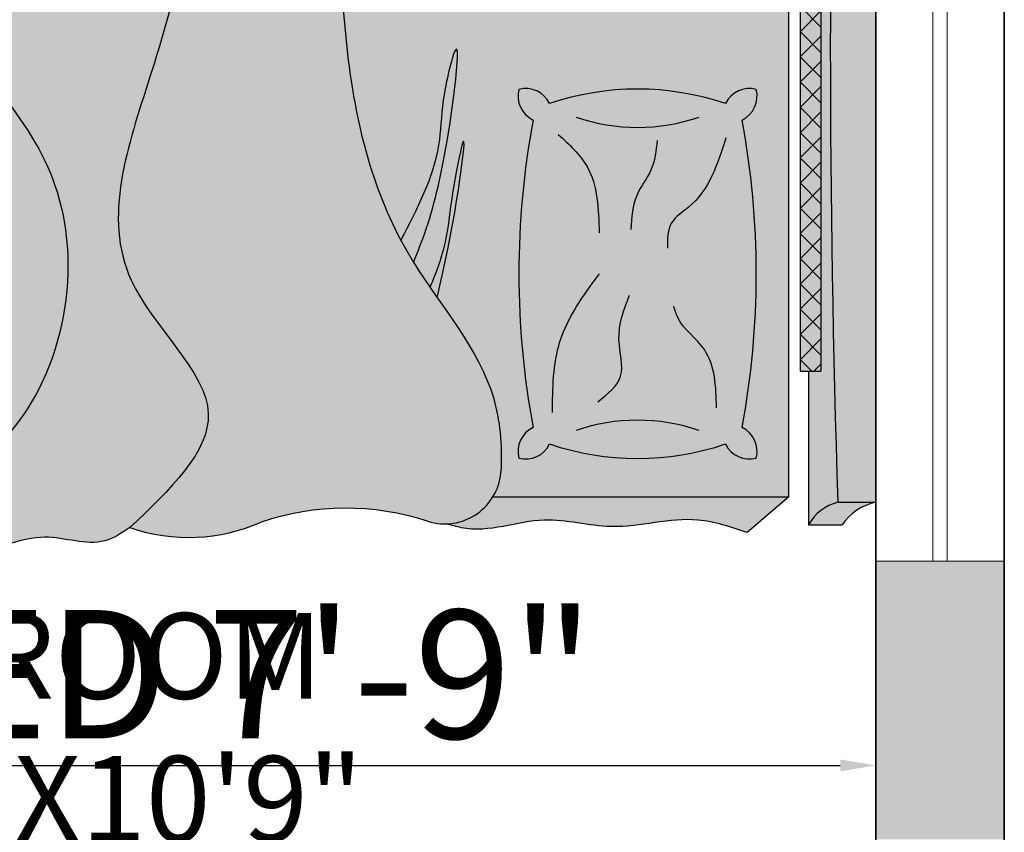
# Model space of a CAD drawing. Units: inches. Extents: x 3148 to 3962, y 1142 to 1671.
# Tile 5 of 9: x 3413 to 3482, y 1426 to 1483. Entities that reach past the tile are written whole.
import ezdxf

# ---------------------------------------------------------------- set-up
doc = ezdxf.new("R2010")
doc.units = ezdxf.units.IN
for name, color, linetype, lineweight in [('A-ANNO-DIMS', 2, 'Continuous', 18), ('A-AREA-IDEN', 7, 'Continuous', 18), ('A-FURN', 8, 'Continuous', 18), ('A-GLAZ', 4, 'Continuous', 18), ('A-WALL', 7, 'Continuous', 35), ('estofado', 7, 'Continuous', 25)]:
    doc.layers.add(name, color=color, linetype=linetype, lineweight=lineweight)
doc.layers.add('A-WALL-PATT', color=252, linetype='Continuous', lineweight=13, true_color=0x939598)
doc.styles.get("Standard").update_dxf_attribs({"font": 'arial.ttf'})
doc.dimstyles.new('ISO-25', dxfattribs={"dimtxt": 9, "dimasz": 2.5, "dimexe": 1.25, "dimexo": 0.625, "dimtad": 1, "dimdec": 1, "dimlunit": 3, "dimtxsty": 'Standard', "dimcen": 2.5, "dimadec": 0, "dimazin": 0, "dimtfac": 1, "dimtdec": 1, "dimtmove": 0, "dimatfit": 3, "dimfxl": 1, "dimarcsym": 0})

# ---------------------------------------------------------------- blocks, each defined once
blk = doc.blocks.new('Cama Box Regencia LOLA')
at = {"layer": 'estofado', "ltscale": 0.2}
h = blk.add_hatch(color=256, dxfattribs=at)
h.dxf.hatch_style = 1
h.set_gradient(color1=(139, 102, 75), color2=(43, 31, 23), one_color=1, tint=0.1299999952316284, name='CURVED')
h.paths.add_polyline_path([(0.8097611300672723, 0), (-0.8097611300671587, 0), (-0.8097611300671587, -0.0676434826297054, 0.0166383680674931), (0.8097611300672723, -0.0676434823212162)])
h = blk.add_hatch(color=256, dxfattribs=at)
h.dxf.hatch_style = 1
h.set_gradient(color1=(139, 102, 75), color2=(43, 31, 23), one_color=1, tint=0.1299999952316284)
h.paths.add_polyline_path([(0.8500000000000227, -0.0600000000000591, -0.1973270565004446), (0.8097611300672723, 0), (0.8097611300672723, -0.0676434826301033, 0.208347730813652), (0.8500000000000227, -0.1199999999998909)])
h = blk.add_hatch(color=256, dxfattribs=at)
h.dxf.hatch_style = 1
h.set_gradient(color1=(139, 102, 75), color2=(43, 31, 23), one_color=1, tint=0.1299999952316284, name='INVCURVED')
h.paths.add_polyline_path([(0.8097611299908749, -0.0676434823237742, -0.0166383680667078), (-0.8097611300671587, -0.0676434826297623, -0.2083477308153697), (-0.8500000000001364, -0.1200000000000045), (-0.5763381074484643, -0.1200000000000045), (-0.5763381074485779, -0.0977075818103117), (0.5763381073808205, -0.0977075818103117), (0.5763381073808205, -0.1200000000000045), (0.8500000000000227, -0.1200000000000045, -0.2083477318100794)])
h = blk.add_hatch(color=256, dxfattribs=at)
h.dxf.hatch_style = 1
h.set_gradient(color1=(139, 102, 75), color2=(198, 169, 149), one_color=1, tint=0.6800000071525574, name='CYLINDER')
h.paths.add_polyline_path([(0.5763381073808205, -0.0977075818103686), (-0.5763381074484643, -0.0977075818103117), (-0.5763381074485779, -0.1348263709859339), (0.5763381073808205, -0.134826370985877)])
h = blk.add_hatch(dxfattribs=at)
h.set_pattern_fill('ANSI37,_O', color=256, scale=0.01)
h.set_pattern_definition([(45, (-24.74368160026529, -44.17612681992631), (-0.0224506403026729, 0.0224506403026729), []), (135, (-24.74368160026529, -44.17612681992631), (-0.0224506403026729, -0.0224506403026729), [])])
h.paths.add_polyline_path([(0.5763381073808205, -0.0977075818103686), (-0.5763381074484643, -0.0977075818103117), (-0.5763381074485779, -0.1348263709859339), (0.5763381073808205, -0.134826370985877)])
h = blk.add_hatch(color=256, dxfattribs=at)
h.dxf.hatch_style = 1
h.set_gradient(color1=(240, 232, 219), color2=(213, 190, 154), one_color=1, tint=0.7200000286102295, name='CURVED')
edge = h.paths.add_edge_path()
edge.add_spline(control_points=[(0.343533776195045, -0.8455058148597345), (0.2879313990920309, -0.8167160606696484), (0.2054770794474052, -0.7744470032542381), (0.0954193394759386, -0.7742416952675626), (-0.0885363502328574, -0.7276964167006668), (0.2428192566063672, -0.7672518992321216), (0.345087521536243, -0.8076697826234067), (0.3825206986321063, -0.8228555492498799)], knot_values=[0.0056315103357428, 0.0056315103357428, 0.0056315103357428, 0.0056315103357428, 0.1860138916206105, 0.2660015162584448, 0.3570871810327863, 0.5963901805690979, 0.739731738908988, 0.739731738908988, 0.739731738908988, 0.739731738908988], degree=3, periodic=0)
edge.add_spline(control_points=[(0.3825206986325611, -0.8228555492497662), (0.3974221570828149, -0.8135511441712424), (0.4121061736600496, -0.8037181558521524), (0.4266849906532571, -0.7937075488799225)], knot_values=[1.358237767273279, 1.358237767273279, 1.358237767273279, 1.358237767273279, 1.409915662372559, 1.409915662372559, 1.409915662372559, 1.409915662372559], degree=3, periodic=0)
edge.add_spline(control_points=[(0.4266849905698109, -0.7937075489369932), (0.3998777739682282, -0.7821381809783361), (0.3476761897024971, -0.7634757898491671), (0.2670618099601825, -0.7565375622627358), (0.0835725072796549, -0.7192994417154637), (0.288524529784695, -0.7446405493717521), (0.4247448861246994, -0.7759943071475277), (0.4449816270193879, -0.7810438091316882)], knot_values=[0.1043639306803623, 0.1043639306803623, 0.1043639306803623, 0.1043639306803623, 0.1896363068641149, 0.2696239315019491, 0.3607095962762907, 0.6000125958126024, 0.6446217338078729, 0.6446217338078729, 0.6446217338078729, 0.6446217338078729], degree=3, periodic=0)
edge.add_spline(control_points=[(0.4449816270197289, -0.7810438091316882), (0.5029779388527232, -0.7406836481117695), (0.5966687145296419, -0.6736247633211292), (0.7071737530245628, -0.6656573253703187), (0.7517012483331201, -0.6672238302253392)], knot_values=[1.43159032281798, 1.43159032281798, 1.43159032281798, 1.43159032281798, 1.63814180148235, 1.770695287284994, 1.770695287284994, 1.770695287284994, 1.770695287284994], degree=3, periodic=0)
edge.add_arc((0.7481853615017826, -0.767162003811734), 0.0999999999999888, 58.7920033978138, 87.98512997550938, ccw=False)
edge.add_line((0.8000000000000682, -0.6816328085782289), (0.8000000000000682, -0.154802362840428))
edge.add_line((0.8000000000000682, -0.154802362840428), (-0.7999999999999546, -0.154802362840428))
edge.add_line((-0.7999999999999546, -0.154802362840428), (-0.8000000000000682, -0.7409839258539819))
edge.add_spline(control_points=[(-0.799999999999841, -0.7409839258539251), (-0.7846451382113174, -0.74846387981205), (-0.7568940913494089, -0.7651582159765554), (-0.7559936909002545, -0.8096905380045313), (-0.7049413305308008, -0.8142555457367848), (-0.7013836936888538, -0.8139988647640733)], knot_values=[0.0122267587020837, 0.0122267587020837, 0.0122267587020837, 0.0122267587020837, 0.0594720782072034, 0.1062176618094138, 0.134458043575382, 0.134458043575382, 0.134458043575382, 0.134458043575382], degree=3, periodic=0)
edge.add_spline(control_points=[(-0.7013836936890812, -0.8139988647637892), (-0.6428309483887916, -0.8132695376718857), (-0.532520673001045, -0.8118955240036598), (-0.2390712668254764, -0.6717984706609172), (-0.3892411364554391, -0.7557901092520752), (-0.4591093260188473, -0.8070101468627512), (-0.5571511178645779, -0.795652750469742), (-0.608497950975675, -0.8409486634728295), (-0.6632498050151981, -0.8266781836207997), (-0.6991149398675134, -0.8254126024436914), (-0.719552182989446, -0.8246914287938125)], knot_values=[0, 0, 0, 0, 0.2187005959148062, 0.4120203559900679, 0.4786136596093368, 0.6046444033330721, 0.6969970394608519, 0.7456449795902803, 0.7925683322559657, 0.8547274388453192, 0.8547274388453192, 0.8547274388453192, 0.8547274388453192], degree=3, periodic=0)
edge.add_spline(control_points=[(-0.7195521829781911, -0.824691428792164), (-0.7293124663336812, -0.8248308281530967), (-0.7545977292818407, -0.8216412233076653), (-0.7742556984202338, -0.794819860189591), (-0.7939222919129634, -0.7820064600295497), (-0.799999999999841, -0.7800193173443404)], knot_values=[0.1564883932805935, 0.1564883932805935, 0.1564883932805935, 0.1564883932805935, 0.184397548386913, 0.2313764834161266, 0.2505984550882281, 0.2505984550882281, 0.2505984550882281, 0.2505984550882281], degree=3, periodic=0)
edge.add_line((-0.8000000000000682, -0.7800193173444541), (-0.7999999999999546, -0.8218505664627286))
edge.add_spline(control_points=[(-0.7999999999999546, -0.8218505664625013), (-0.7938082505512511, -0.8290217081292894), (-0.7673857405620766, -0.8512914803976059), (-0.7619109683460011, -0.8661369353891359), (-0.6555700939965164, -0.8510070218793543), (-0.7139793977868294, -0.8637526923380391), (-0.7379026254519659, -0.8623504601624176), (-0.7688129786438367, -0.8813042143888196), (-0.7854260296310259, -0.8561610219318254), (-0.7961930533253962, -0.8566031243811949), (-0.7999999999999546, -0.8573491405791173)], knot_values=[0.0595743221876141, 0.0595743221876141, 0.0595743221876141, 0.0595743221876141, 0.08075289116965, 0.1037414994169835, 0.1697200936249022, 0.1760361327243865, 0.2071371586311508, 0.2404744334261798, 0.2623408547027293, 0.2736604507987723, 0.2736604507987723, 0.2736604507987723, 0.2736604507987723], degree=3, periodic=0)
edge.add_line((-0.7999999999999546, -0.8573491405791173), (-0.8000000000000682, -0.9113562424721521))
edge.add_spline(control_points=[(-0.8000000000000682, -0.9113562424720385), (-0.7937204054647964, -0.9077594990848183), (-0.7710343135782978, -0.8978798065321029), (-0.7213062468074442, -0.9144666877443228), (-0.6268586829058905, -0.862430497409548), (-0.6896594748232019, -0.9045634991654196), (-0.7483442493064559, -0.9189273406958591), (-0.7835301183422417, -0.922920432793262), (-0.7896301351460125, -0.9477657000142585), (-0.7975786973822779, -0.955260590410262), (-0.8000000000001818, -0.9571831923294098)], knot_values=[0.0138560263374175, 0.0138560263374175, 0.0138560263374175, 0.0138560263374175, 0.0348737775836104, 0.0888666909546002, 0.1078792274429341, 0.1267378491223226, 0.1587140219647659, 0.1937574699451985, 0.2174867851300671, 0.2267221218327879, 0.2267221218327879, 0.2267221218327879, 0.2267221218327879], degree=3, periodic=0)
edge.add_line((-0.7999999999999546, -0.957183192329296), (-0.7999999999999546, -1.145824641594742))
edge.add_spline(control_points=[(-0.8000000000002955, -1.145824641594913), (-0.7271039467997298, -1.094596787649038), (-0.4885706936571524, -0.9465888221489535), (-0.0701640902225336, -0.9707493165000187), (0.237911901821235, -0.902164522332157), (0.3435337762145991, -0.845505814843193)], knot_values=[0.1168958193629841, 0.1168958193629841, 0.1168958193629841, 0.1168958193629841, 0.3797203297758731, 0.9577018633805092, 1.31379338443587, 1.31379338443587, 1.31379338443587, 1.31379338443587], degree=3, periodic=0)
h.paths.add_polyline_path([(-0.6766340706021765, -0.6101327540145576, -0.3575266660906883), (-0.7312746368313583, -0.6354535276154252, -0.3575266660894137), (-0.7059538632299791, -0.5808129613865844, -0.1647847126465284), (-0.7059538632300928, -0.2676124402649407, -0.3575266660890756), (-0.7312746368312446, -0.2129718740360431, -0.3575266660908716), (-0.6766340706020629, -0.2382926476369676, -0.0925607043966334), (-0.1295169377724505, -0.2382926476369107, -0.3575266660898965), (-0.0748763715433825, -0.2129718740360431, -0.3575266660894428), (-0.1001971451446479, -0.2676124402649407, -0.1647847126465285), (-0.1001971451445343, -0.5808129613865844, -0.3575266660890756), (-0.0748763715433825, -0.6354535276154821, -0.3575266660898962), (-0.1295169377724505, -0.6101327540146145, -0.0925607043966531)], flags=16)
h.paths.add_polyline_path([(0.0748763715433825, -0.6354535276157094, -0.3575266660910266), (0.1001971451446479, -0.5808129613865844, -0.1647847126465284), (0.1001971451445343, -0.2676124402649407, -0.3575266660890757), (0.0748763715433825, -0.2129718740360431, -0.3575266660898962), (0.1295169377724505, -0.2382926476369107, -0.0925607043966334), (0.6766340706020629, -0.2382926476369676, -0.3575266660908718), (0.7312746368312446, -0.2129718740360431, -0.3575266660894425), (0.7059538632299791, -0.2676124402649407, -0.1647847126465283), (0.7059538632300928, -0.5808129613865844, -0.3575266660890756), (0.7312746368312446, -0.6354535276154821, -0.3575266660908716), (0.6766340706020629, -0.6101327540145576, -0.0925607043966335), (0.1295169377724505, -0.6101327540146145, -0.3575266660906303)], flags=16)
h = blk.add_hatch(color=256, dxfattribs=at)
h.dxf.hatch_style = 1
h.set_gradient(color1=(240, 232, 219), color2=(213, 190, 154), one_color=1, tint=0.7200000286102295)
edge = h.paths.add_edge_path()
edge.add_spline(control_points=[(0.8481164014890509, -0.7634488855285327), (0.8506728373771466, -0.7550468983013161), (0.868679602201837, -0.6953776187201015), (0.8253488717913342, -0.6001498518888299), (0.8674912876568897, -0.4595932758330151), (0.8269013755603964, -0.3369378214810581), (0.8537222782124445, -0.258285373872468), (0.8635971996978923, -0.2293271111754507)], knot_values=[0, 0, 0, 0, 0.0246217641678395, 0.1732110090087366, 0.2929197011275091, 0.4476746021509216, 0.5378548332073604, 0.5378548332073604, 0.5378548332073604, 0.5378548332073604], degree=3, periodic=0)
edge.add_line((0.8635971996978923, -0.229327111175337), (0.8000000000001818, -0.1548023628403712))
edge.add_line((0.8000000000001818, -0.1548023628403712), (0.8000000000000682, -0.681632808574193))
edge.add_arc((0.7481853615026921, -0.7671620038083234), 0.0999999999999888, 2.1279492292164264, 58.79200339844499, ccw=False)
h = blk.add_hatch(color=256, dxfattribs=at)
h.dxf.hatch_style = 1
h.set_gradient(color1=(106, 82, 42), color2=(160, 123, 64), one_color=1, tint=0.4399999976158142, name='CURVED')
h.paths.add_polyline_path([(0.7059538632300928, -0.2676124402650544, 0.3575266660910843), (0.731274636831131, -0.2129718740358157, 0.3575266660898384), (0.6766340706021765, -0.2382926476369107, 0.092560704396653), (0.1295169377724505, -0.2382926476369676, 0.3575266660900799), (0.0748763715433825, -0.2129718740360431, 0.3575266660883129), (0.1001971451444206, -0.2676124402648838, 0.1647847126464969), (0.1001971451445343, -0.5808129613864708, 0.3575266660914516), (0.0748763715433825, -0.6354535276157094, 0.3575266660906303), (0.1295169377724505, -0.6101327540146145, 0.0925607043966335), (0.6766340706020629, -0.6101327540146145, 0.3575266660906881), (0.7312746368312446, -0.6354535276154821, 0.3575266660886796), (0.7059538632300928, -0.5808129613866413, 0.1647847126464968)])
h = blk.add_hatch(color=256, dxfattribs=at)
h.dxf.hatch_style = 1
h.set_gradient(color1=(206, 178, 131), color2=(227, 212, 186), one_color=1, tint=0.8100000023841857, name='CYLINDER')
edge = h.paths.add_edge_path()
edge.add_arc((0.7481853614966667, -0.7671620038115634), 0.0999999999999888, 342.0511336145294, 447.9851299725766)
edge.add_spline(control_points=[(0.7517012483331201, -0.6672238302253392), (0.7071737530245628, -0.6656573253703187), (0.5966687145298692, -0.6736247633211292), (0.5029779388527232, -0.7406836481117125), (0.4449816270195015, -0.7810438091316314)], knot_values=[1.431590322817835, 1.431590322817835, 1.431590322817835, 1.431590322817835, 1.564143808620479, 1.770695287284994, 1.770695287284994, 1.770695287284994, 1.770695287284994], degree=3, periodic=0)
edge.add_spline(control_points=[(0.4449816270195015, -0.7810438091316314), (0.4388957332065502, -0.7852790380018178), (0.4327996148541616, -0.7895089160493285), (0.4266849906533708, -0.7937075488798087)], knot_values=[1.409915662372814, 1.409915662372814, 1.409915662372814, 1.409915662372814, 1.431590322817835, 1.431590322817835, 1.431590322817835, 1.431590322817835], degree=3, periodic=0)
edge.add_spline(control_points=[(0.4266849906533708, -0.7937075488798087), (0.4121061736600496, -0.8037181558521524), (0.3974221570825875, -0.8135511441712991), (0.38252069863222, -0.8228555492498799)], knot_values=[1.358237767273037, 1.358237767273037, 1.358237767273037, 1.358237767273037, 1.409915662372815, 1.409915662372815, 1.409915662372815, 1.409915662372815], degree=3, periodic=0)
edge.add_line((0.3825206986330158, -0.8228555492493114), (0.343533776286904, -0.8455058148063584))
edge.add_spline(control_points=[(0.3435337761924302, -0.8455058148550165), (0.2379119018048641, -0.902164522335795), (-0.0701640902311738, -0.9707493164995071), (-0.4885706936571524, -0.9465888221488967), (-0.7271039467997298, -1.094596787649038), (-0.8000000000000682, -1.145824641594742)], knot_values=[0.1168958193630798, 0.1168958193630798, 0.1168958193630798, 0.1168958193630798, 0.472987340393773, 1.050968873998409, 1.313793384411202, 1.313793384411202, 1.313793384411202, 1.313793384411202], degree=3, periodic=0)
edge.add_spline(control_points=[(-0.8000000000000682, -1.145824641594742), (-0.8038896190357718, -1.14855807951244), (-0.8077744942224853, -1.151305646504738), (-0.8116551946761774, -1.154065647517199)], knot_values=[0.1028719158199011, 0.1028719158199011, 0.1028719158199011, 0.1028719158199011, 0.1168958193630799, 0.1168958193630799, 0.1168958193630799, 0.1168958193630799], degree=3, periodic=0)
edge.add_arc((-0.7536973518524519, -1.235557294053705), 0.1000000000000352, 125.4208969883762, 169.6981795679068)
edge.add_spline(control_points=[(-0.852085287466366, -1.217673946333093), (-0.8521399740518518, -1.217974812833915), (-0.8565649010855622, -1.242328483616745), (-0.8662697220019026, -1.297321141147904), (-0.8487158298532904, -1.34896742172242), (-0.8348745804664758, -1.381844109035796)], knot_values=[0.3128349436863077, 0.3128349436863077, 0.3128349436863077, 0.3128349436863077, 0.3137509534211996, 0.386958004641742, 0.4759027329026081, 0.4759027329026081, 0.4759027329026081, 0.4759027329026081], degree=3, periodic=0)
edge.add_spline(control_points=[(-0.8348745804664758, -1.38184410903591), (-0.8226532004149476, -1.367823298399059), (-0.8056354908857201, -1.352141651537124), (-0.7460155199962628, -1.32170802000337)], knot_values=[0.0062456970656236, 0.0062456970656236, 0.0062456970656236, 0.0062456970656236, 0.0554759259147193, 0.0554759259147193, 0.0554759259147193, 0.0554759259147193], degree=3, periodic=0)
edge.add_spline(control_points=[(-0.7460155200169539, -1.321708019985464), (-0.6188339616464873, -1.25080943574278), (-0.3488365122128698, -1.179158668568902), (0.0338148848931041, -1.279726484458706), (0.3977250465933366, -1.412092721352792), (0.6449024721503065, -1.106270719748692), (0.7873766543807506, -1.256744909425322), (0.8547271521993025, -1.327877176513538)], knot_values=[0.0991852523588446, 0.0991852523588446, 0.0991852523588446, 0.0991852523588446, 0.5236467270390676, 0.9270872950244264, 1.289918234564769, 1.564439021262726, 1.810554634340498, 1.810554634340498, 1.810554634340498, 1.810554634340498], degree=3, periodic=0)
edge.add_arc((0.5509678495186563, -1.223443291813453), 0.3212104454069235, 341.0267878798241, 383.7782184284114)
edge.add_arc((1.292676354991499, -0.9435407756057543), 0.4723459732861395, 162.0511336103901, 198.5657216587827, ccw=False)
h = blk.add_hatch(color=256, dxfattribs=at)
h.dxf.hatch_style = 1
h.set_gradient(color1=(240, 232, 219), color2=(137, 106, 57), one_color=1, tint=0.3799999952316284, name='CURVED')
edge = h.paths.add_edge_path()
edge.add_spline(control_points=[(0.3825206986321063, -0.8228555492498799), (0.345087521536243, -0.8076697826234067), (0.2428192566063672, -0.7672518992321216), (-0.0885363502328574, -0.7276964167006668), (0.0954193394759386, -0.7742416952675626), (0.2054770794474052, -0.7744470032542381), (0.2879313990920309, -0.8167160606696484), (0.343533776195045, -0.8455058148597345)], knot_values=[0.0056315103357428, 0.0056315103357428, 0.0056315103357428, 0.0056315103357428, 0.1489730686756328, 0.3882760682119444, 0.479361732986286, 0.5593493576241202, 0.739731738908988, 0.739731738908988, 0.739731738908988, 0.739731738908988], degree=3, periodic=0)
edge.add_line((0.343533776195045, -0.8455058148597913), (0.3825206986321063, -0.8228555492498799))
h = blk.add_hatch(color=256, dxfattribs=at)
h.dxf.hatch_style = 1
h.set_gradient(color1=(240, 232, 219), color2=(137, 106, 57), one_color=1, tint=0.3799999952316284, name='CURVED')
edge = h.paths.add_edge_path()
edge.add_spline(control_points=[(0.4449816270193879, -0.7810438091316882), (0.4247448861246994, -0.7759943071475277), (0.288524529784695, -0.7446405493717521), (0.0835725072796549, -0.7192994417154637), (0.2670618099601825, -0.7565375622627358), (0.3476761897024971, -0.7634757898491671), (0.3998777739682282, -0.7821381809783361), (0.4266849905698109, -0.7937075489369932)], knot_values=[0.1043639306803623, 0.1043639306803623, 0.1043639306803623, 0.1043639306803623, 0.1489730686756328, 0.3882760682119444, 0.479361732986286, 0.5593493576241202, 0.6446217338078729, 0.6446217338078729, 0.6446217338078729, 0.6446217338078729], degree=3, periodic=0)
edge.add_spline(control_points=[(0.4266849906528023, -0.7937075488800929), (0.4327996148537068, -0.7895089160495559), (0.4388957332062092, -0.7852790380020452), (0.4449816270192742, -0.781043809131802)], knot_values=[1.409915662372559, 1.409915662372559, 1.409915662372559, 1.409915662372559, 1.43159032281798, 1.43159032281798, 1.43159032281798, 1.43159032281798], degree=3, periodic=0)
h = blk.add_hatch(color=256, dxfattribs=at)
h.dxf.hatch_style = 1
h.set_gradient(color1=(206, 178, 131), color2=(233, 221, 200), one_color=1, tint=0.8500000238418579, name='CURVED')
edge = h.paths.add_edge_path()
edge.add_spline(control_points=[(0.9233883396182136, -2.254908822900802), (0.9143712174658276, -2.237158585978875), (0.8971704820246486, -2.20329887728792), (0.9295105801843419, -2.140290914518345), (0.848651568119294, -2.10957861148239), (0.9047062348403186, -2.046222426005954), (0.8299480774321636, -1.990932361540615), (0.9387479200587449, -1.92692496801726), (0.8590435458045249, -1.86767849203585), (0.8322262745575699, -1.826028043643361), (0.8247981799574972, -1.810442049687992)], knot_values=[0, 0, 0, 0, 0.0575832900035364, 0.1098437972159638, 0.1698138218664432, 0.2255174829302509, 0.2824861515521905, 0.3632291183773252, 0.4509842065695901, 0.5012091817853866, 0.5012091817853866, 0.5012091817853866, 0.5012091817853866], degree=3, periodic=0)
edge.add_spline(control_points=[(0.8247981799572698, -1.810442049688447), (0.8512430237993839, -1.769990096378137), (0.8869160776755506, -1.705010622333873), (0.9070359522544322, -1.586338752195842), (0.8536462472426364, -1.488247672851343), (0.8944567470317679, -1.387739666353695), (0.8643796102055603, -1.342420998864781), (0.8547271521993025, -1.327877176513538)], knot_values=[0, 0, 0, 0, 0.1438744691785906, 0.2224893870322766, 0.3492927143212738, 0.4561786976395368, 0.5066917301592304, 0.5066917301592304, 0.5066917301592304, 0.5066917301592304], degree=3, periodic=0)
edge.add_spline(control_points=[(0.8547271521993025, -1.327877176513538), (0.7873766543807506, -1.256744909425322), (0.6449024721503065, -1.106270719748692), (0.3977250465933366, -1.412092721352792), (0.0338148848931041, -1.279726484458706), (-0.3488365122128698, -1.179158668568902), (-0.6188339616464873, -1.25080943574278), (-0.7460155200169539, -1.321708019985464)], knot_values=[0.0991852523588446, 0.0991852523588446, 0.0991852523588446, 0.0991852523588446, 0.3453008654366167, 0.6198216521345741, 0.9826525916749167, 1.386093159660275, 1.810554634340498, 1.810554634340498, 1.810554634340498, 1.810554634340498], degree=3, periodic=0)
edge.add_spline(control_points=[(-0.7460155199962628, -1.32170802000337), (-0.8056354908857201, -1.352141651537124), (-0.8226532004149476, -1.367823298399059), (-0.8348745804664758, -1.38184410903591)], knot_values=[0.0062456970656236, 0.0062456970656236, 0.0062456970656236, 0.0062456970656236, 0.0554759259147193, 0.0554759259147193, 0.0554759259147193, 0.0554759259147193], degree=3, periodic=0)
edge.add_spline(control_points=[(-0.8348745804664758, -1.38184410903591), (-0.8364250716851984, -1.383622888820184), (-0.8378983647115774, -1.385374937005849), (-0.8393716577378427, -1.387126985191514)], knot_values=[0, 0, 0, 0, 0.0062456970656236, 0.0062456970656236, 0.0062456970656236, 0.0062456970656236], degree=3, periodic=0)
edge.add_arc((-0.6180450437709624, -1.576392779500167), 0.2912164331649039, 139.4648411061637, 203.3711573294546)
edge.add_arc((-0.7011750866292914, -1.609837078845487), 0.2016528082906132, 204.0179006417974, 212.6189639884946)
edge.add_spline(control_points=[(-0.8710220093900034, -1.718537943240505), (-0.8696870122217887, -1.721658691442996), (-0.8597709916446092, -1.746046247230935), (-0.8464685798230674, -1.804421032451443), (-0.888988689927828, -1.889951451602371), (-0.8378676506146121, -1.973422824210047), (-0.8371590179440318, -2.05992368952792), (-0.8871569320951948, -2.144598622072578), (-0.908935644436724, -2.210906123939594), (-0.9233883398977695, -2.254908823284267)], knot_values=[0, 0, 0, 0, 0.0101500649009363, 0.0785829584511912, 0.1732273504791735, 0.2688802694005398, 0.3498050162211252, 0.4202002266429896, 0.5590752189863636, 0.5590752189863636, 0.5590752189863636, 0.5590752189863636], degree=3, periodic=0)
edge.add_ellipse((-0.9040800600764669, -2.258882422916315), major_axis=(0.0267880171833212, 0.0267880171833213), ratio=0.4535320972039226, start_angle=94.15910660291303, end_angle=123.37101895145429, ccw=False)
edge.add_ellipse((-0.8772920428931456, -2.232094405732993), major_axis=(0.0772920428927364, 0.0772920428927364), ratio=0.168252450050839, start_angle=-1.0527401173021644e-10, end_angle=156.3071135567154, ccw=False)
edge.add_line((-0.8000000000002955, -2.154802362840428), (0.7999592378284888, -2.154802362840428))
edge.add_arc((0.9462065466516378, -2.098298447668867), 0.1567831871334379, 200.9447658774159, 201.1244713640487, ccw=False)
edge.add_arc((1.115979327553759, -2.004946707326951), 0.3497136727815615, 205.2898146244752, 205.3730108333857)
edge.add_ellipse((0.8772920428930319, -2.232094405732993), major_axis=(-0.0772920428927364, 0.0772920428927364), ratio=0.168252450050839, start_angle=203.6928864432847, end_angle=359.99999999994674, ccw=False)
edge.add_ellipse((0.9040800600763532, -2.258882422916315), major_axis=(-0.0267880171833213, 0.0267880171833213), ratio=0.4535320972039226, start_angle=236.6289810485458, end_angle=265.84089339708703, ccw=False)
for p, q in [((0.8097611300672723, -0.0676434826300465), (0.8097611300672723, 0)), ((-0.5763381074485779, -0.0977075818103686), (0.5763381073808205, -0.0977075818103686)), ((0.5763381073808205, -0.1348263709859339), (0.5763381073808205, -0.0977075818103686)), ((-0.5763381074485779, -0.1348263709859339), (0.5763381073808205, -0.1348263709859339)), ((0.8000000000000682, -0.154802362840428), (0.8635971996978923, -0.2293271111754507)), ((0.3825206986321063, -0.8228555492498799), (0.343533776195045, -0.8455058148597913))]:
    blk.add_line(p, q, dxfattribs=at)
for points in [[(0.8097611300672723, 0), (-0.8097611300671587, 0)], [(0.5763381073808205, -0.1200000000000045), (0.8500000000000227, -0.1200000000000045), (0.8500000000000227, -0.0600000000000591)], [(0.8000000000000682, -0.6816328085741361), (0.8000000000000682, -0.154802362840428), (-0.7999999999999546, -0.154802362840428), (-0.7999999999999546, -0.7409839258540956)]]:
    blk.add_lwpolyline(points, dxfattribs=at)
for centre, radius, start, end in [((0.9029365906353632, 0.0189948651997156), 0.0950919100450938, 191.5224976221414, 236.1728936464908), ((-4.6343303e-09, 24.25977121121599), 24.3408877974203, 268.0935593847751, 271.9064406368756), ((0.8899769538815007, -0.0476343534641615), 0.0826737179530018, 194.0061042842989, 241.0824226245542), ((0.120860229745972, -0.2248498560688859), 0.047493175008304, 165.516646303857, 244.209945069049), ((0.0867543535765663, -0.2589557322385758), 0.047493175008304, 25.79005493108792, 104.4833536962803), ((0.4030755041873136, -1.703357436968531), 1.490385562932656, 79.42346065608726, 100.5765393439197), ((0.7193966547980608, -0.2589557322385758), 0.047493175008304, 75.51664630371964, 154.2099450689121), ((0.6852907786285414, -0.2248498560688859), 0.047493175008304, 295.790054930951, 14.48335369614292), ((0.562460708312642, -0.4242127008258194), 0.4880688921049917, 161.2852469077218, 198.7147530922607), ((0.243690300061985, -0.4242127008258194), 0.4880688921049917, 341.2852469077393, 18.71475309227822), ((-0.19631084963396, -0.4242127008257626), 0.3387897965243698, 341.1598423418016, 18.84015765820971), ((1.002461858008359, -0.4242127008257626), 0.3387897965243698, 161.1598423417902, 198.8401576581983), ((0.120860229745972, -0.6235755455826393), 0.047493175008304, 115.790054930951, 194.4833536961429), ((0.6852907786285414, -0.6235755455826393), 0.047493175008304, 345.516646303857, 64.20994506904903), ((0.0867543535765663, -0.5894696694129494), 0.047493175008304, 255.5166463037197, 334.2099450689121), ((0.4030755041873136, 0.8549320353169491), 1.490385562932656, 259.4234606560803, 280.5765393439127), ((0.7193966547980608, -0.5894696694129494), 0.047493175008304, 205.7900549310879, 284.4833536962804), ((0.7481853615029195, -0.7671620038083234), 0.1, 342.0511336116027, 87.98512997616182), ((1.292676354991613, -0.9435407756055268), 0.4723459732861117, 162.0511336104213, 198.5657216589983), ((0.55096784951877, -1.223443291813453), 0.3212104454069235, 341.0267878798186, 23.77821842812888)]:
    blk.add_arc(centre, radius, start, end, dxfattribs=at)
for points, knots in [([(0.8635971996978923, -0.2293271111754507), (0.8537222782124445, -0.258285373872468), (0.8269013755603964, -0.3369378214810581), (0.8674912876568897, -0.4595932758330151), (0.8253488717913342, -0.6001498518888299), (0.868679602201837, -0.6953776187201015), (0.8506728373771466, -0.7550468983013161), (0.8481164014890509, -0.7634488855285327)], [0, 0, 0, 0, 0.0901802310564388, 0.2449351320798513, 0.3646438241986237, 0.5132330690395209, 0.5378548332073604, 0.5378548332073604, 0.5378548332073604, 0.5378548332073604]), ([(0.1609929429250769, -0.2668120520876869), (0.207361296664481, -0.2816189425177519), (0.2673465842344797, -0.3007741531050562), (0.3100088172549912, -0.3711986237053177), (0.3410959220547441, -0.371113456673647), (0.3573768361287648, -0.371068853062809)], [0, 0, 0, 0, 0.1404794637529129, 0.1817338842404631, 0.2270973195475621, 0.2270973195475621, 0.2270973195475621, 0.2270973195475621]), ([(0.641547568925148, -0.2836087781224137), (0.6039704843628328, -0.2846768301159754), (0.539944686002343, -0.2864966328594507), (0.4983244357833337, -0.3487001107148991), (0.4673537235191868, -0.3577134183149331), (0.460449429265168, -0.3597227530484019)], [0, 0, 0, 0, 0.1057518620258909, 0.1801855432155129, 0.2015394496060149, 0.2015394496060149, 0.2015394496060149, 0.2015394496060149]), ([(0.1657269282603693, -0.3891622340328808), (0.1839821155447316, -0.3912290170364152), (0.2191851220416109, -0.3952145677934529), (0.2641538569791404, -0.4324302667024541), (0.3028411853428648, -0.4348886966416372), (0.3243911361614664, -0.4362581125853354)], [0, 0, 0, 0, 0.0540396012867365, 0.1042090889319622, 0.1672963371706364, 0.1672963371706364, 0.1672963371706364, 0.1672963371706364]), ([(0.630774277431101, -0.4946666993113809), (0.6169895699779718, -0.4772535648042688), (0.5885015945383536, -0.441266950663047), (0.5131074616321869, -0.4662255111125919), (0.4667910825139399, -0.4484404284426592), (0.4408934738504513, -0.4384959742387196)], [0, 0, 0, 0, 0.0606588350328579, 0.1253597443752535, 0.2074214353097695, 0.2074214353097695, 0.2074214353097695, 0.2074214353097695]), ([(0.1552772464440295, -0.5652394970176715), (0.1730924483668451, -0.5457941389807961), (0.2188221854511549, -0.4958799637506091), (0.2880058022633399, -0.4937226941133118), (0.3302371516485891, -0.4924058446629829)], [0, 0, 0, 0, 0.0765478869158952, 0.1964903209174588, 0.1964903209174588, 0.1964903209174588, 0.1964903209174588]), ([(0.6501439432536245, -0.5758072434303472), (0.6067249420939599, -0.5753127958675333), (0.5155219215609228, -0.5742741927209986), (0.4416129136043037, -0.5203678897559305), (0.402889750189047, -0.4921247481343585)], [0, 0, 0, 0, 0.1270530108164939, 0.2668789710677518, 0.2668789710677518, 0.2668789710677518, 0.2668789710677518]), ([(0.38252069863222, -0.8228555492498799), (0.4632317710900225, -0.7724599107979202), (0.5727651217678158, -0.6753482176968646), (0.7071737530245628, -0.6656573253703187), (0.7517012483331201, -0.6672238302253392)], [1.358237767273037, 1.358237767273037, 1.358237767273037, 1.358237767273037, 1.63814180148235, 1.770695287284994, 1.770695287284994, 1.770695287284994, 1.770695287284994]), ([(0.3825206986321063, -0.8228555492498799), (0.345087521536243, -0.8076697826234067), (0.2428192566063672, -0.7672518992321216), (-0.0885363502328574, -0.7276964167006668), (0.0954193394759386, -0.7742416952675626), (0.2054770794474052, -0.7744470032542381), (0.2879313990920309, -0.8167160606696484), (0.343533776195045, -0.8455058148597345)], [0.0056315103357428, 0.0056315103357428, 0.0056315103357428, 0.0056315103357428, 0.1489730686756328, 0.3882760682119444, 0.479361732986286, 0.5593493576241202, 0.739731738908988, 0.739731738908988, 0.739731738908988, 0.739731738908988]), ([(0.4449816270193879, -0.7810438091316882), (0.4247448861246994, -0.7759943071475277), (0.288524529784695, -0.7446405493717521), (0.0835725072796549, -0.7192994417154637), (0.2670618099601825, -0.7565375622627358), (0.3476761897024971, -0.7634757898491671), (0.3998777739682282, -0.7821381809783361), (0.4266849905698109, -0.7937075489369932)], [0.1043639306803623, 0.1043639306803623, 0.1043639306803623, 0.1043639306803623, 0.1489730686756328, 0.3882760682119444, 0.479361732986286, 0.5593493576241202, 0.6446217338078729, 0.6446217338078729, 0.6446217338078729, 0.6446217338078729]), ([(-0.8116551946761774, -1.154065647517199), (-0.7350455857787211, -1.099579968801037), (-0.493473113061782, -0.9463057365681493), (-0.0701640902311738, -0.9707493164995071), (0.2379119018048641, -0.902164522335795), (0.3435337761924302, -0.8455058148550165)], [0.1028719158199011, 0.1028719158199011, 0.1028719158199011, 0.1028719158199011, 0.3797203297758731, 0.9577018633805092, 1.313793384411202, 1.313793384411202, 1.313793384411202, 1.313793384411202]), ([(-0.7460155200169539, -1.321708019985464), (-0.6188339616464873, -1.25080943574278), (-0.3488365122128698, -1.179158668568902), (0.0338148848931041, -1.279726484458706), (0.3977250465933366, -1.412092721352792), (0.6449024721503065, -1.106270719748692), (0.7873766543807506, -1.256744909425322), (0.8547271521993025, -1.327877176513538)], [0.0991852523588446, 0.0991852523588446, 0.0991852523588446, 0.0991852523588446, 0.5236467270390676, 0.9270872950244264, 1.289918234564769, 1.564439021262726, 1.810554634340498, 1.810554634340498, 1.810554634340498, 1.810554634340498]), ([(0.8547271521993025, -1.327877176513538), (0.8643796102055603, -1.342420998864781), (0.8944567470317679, -1.387739666353695), (0.8536462472426364, -1.488247672851343), (0.9070359522544322, -1.586338752195842), (0.8869160776755506, -1.705010622333873), (0.8512430237993839, -1.769990096378137), (0.8247981799572698, -1.810442049688447)], [0, 0, 0, 0, 0.0505130325196935, 0.1573990158379565, 0.2842023431269537, 0.3628172609806397, 0.5066917301592304, 0.5066917301592304, 0.5066917301592304, 0.5066917301592304]), ([(-0.8337777191962914, -1.686127396833001), (-0.7936227331957753, -1.590003258421234), (-0.5563859991466416, -1.394748990587913), (-0.1321102153461879, -1.783182047565389), (0.1908245506583626, -1.429131816234075), (0.5373208507353411, -1.424480211867205), (0.720102724937533, -1.549855593291283), (0.836774155394778, -1.71068108627179)], [0.0299011711635954, 0.0299011711635954, 0.0299011711635954, 0.0299011711635954, 0.2769669118207226, 0.7971145189980146, 1.093669199334649, 1.464665995707328, 1.788488893467898, 1.788488893467898, 1.788488893467898, 1.788488893467898])]:
    blk.add_open_spline(points, degree=3, knots=knots, dxfattribs=at)
blk = doc.blocks.new('WIN-72')
for p, q in [((0.0003062757873522, 72.00020003451709), (9.000306275787352, 72.00020003451709)), ((4.000306275787352, 72.00020003451687), (4.000306275788716, 0.0002000345168653)), ((5.000306275787352, 72.00020003451687), (5.000306275788716, 0.0002000345168653)), ((0.0003062757873522, 0.0002000345170927), (9.000306275787352, 0.0002000345170927))]:
    blk.add_line(p, q)
blk = doc.blocks.new('*D94')
at = {"layer": 'A-ANNO-DIMS', "color": 0, "lineweight": -2, "transparency": 16777216}
for p, q in [((3379.971676630814, 1444.320308753911), (3379.971676630814, 1429.734714307165)), ((3473.042306275787, 1444.320308753911), (3473.042306275787, 1429.734714307165)), ((3382.471676630814, 1430.984714307166), (3470.542306275787, 1430.984714307166))]:
    blk.add_line(p, q, dxfattribs=at)
at = {"layer": 'A-ANNO-DIMS', "color": 0, "transparency": 16777216}
for points in [[(3382.471676630814, 1431.401380973832), (3382.471676630814, 1430.568047640499), (3379.971676630814, 1430.984714307166)], [(3470.542306275787, 1431.401380973832), (3470.542306275787, 1430.568047640499), (3473.042306275787, 1430.984714307166)]]:
    blk.add_solid(points, dxfattribs=at)
at = {"layer": 'Defpoints', "color": 0, "transparency": 16777216}
for p in [(3379.971676630814, 1444.945308753911), (3473.042306275787, 1444.945308753911), (3473.042306275787, 1430.984714307166)]:
    blk.add_point(p, dxfattribs=at)
at = {"layer": 'A-ANNO-DIMS', "color": 0, "transparency": 16777216, "insert": (3426.506991453301, 1436.204871196661), "char_height": 9, "attachment_point": 5}
blk.add_mtext('BED 7\'-9"', dxfattribs=at)

msp = doc.modelspace()

# ---------------------------------------------------------------- hatches: boundary and pattern name
at = {"layer": 'A-WALL-PATT'}
h = msp.add_hatch(color=256, dxfattribs=at)
h.dxf.hatch_style = 1
h.paths.add_polyline_path([(3203.042306275788, 1410.799200034518), (3194.042306275787, 1410.799200034518), (3194.042306275787, 1296.799200034517), (3203.042306275786, 1296.799200034517), (3203.042306275787, 1300.855382799943)])
h.paths.add_polyline_path([(3203.042306275778, 1281.799200034517), (3194.042306275787, 1281.799200034517), (3194.042306275787, 1212.799200034517), (3203.042306275788, 1212.799200034517)])
h.paths.add_polyline_path([(3326.042306275788, 1206.799200034517), (3203.042306275788, 1206.799200034517), (3203.042306275788, 1197.799200034517), (3326.042306275788, 1197.799200034517)])
h.paths.add_polyline_path([(3341.042306275787, 1362.799200034517), (3335.042306275788, 1362.799200034517), (3335.042306275788, 1290.799200034517), (3341.042306275787, 1290.799200034517)])
h.paths.add_polyline_path([(3341.042306275788, 1207.799200034517), (3335.042306275788, 1207.799200034517), (3335.042306275788, 1206.799200034517), (3341.042306275788, 1206.799200034517)])
h.paths.add_polyline_path([(3341.042306275787, 1259.799200034517), (3335.042306275788, 1259.799200034517), (3335.042306275788, 1255.799200034517), (3341.042306275787, 1255.799200034517)])
h.paths.add_polyline_path([(3341.042306275787, 1281.799200034517), (3335.042306275788, 1281.799200034517), (3335.042306275788, 1277.799200034517), (3341.042306275787, 1277.799200034517)])
h.paths.add_polyline_path([(3377.042306275787, 1287.799200034517), (3350.042306275788, 1287.799200034517), (3350.042306275788, 1281.799200034517), (3377.042306275787, 1281.799200034517)])
h.paths.add_polyline_path([(3473.042306275787, 1287.799200034517), (3445.042307275787, 1287.799200034517), (3437.042306275787, 1287.799200034517), (3437.042306275788, 1281.799200034517), (3473.042306275787, 1281.799200034517)])
h.paths.add_polyline_path([(3482.042306275788, 1313.299200034517), (3473.042306275787, 1313.299200034517), (3473.042306275787, 1296.799200034517), (3482.042306275788, 1296.799200034517)])
h.paths.add_polyline_path([(3482.042306275788, 1410.799200034517), (3473.042306275787, 1410.799200034517), (3473.042306275787, 1385.299200034517), (3482.042306275788, 1385.299200034517)])
h.paths.add_polyline_path([(3473.042306275787, 1416.799200034517), (3344.042306275788, 1416.799200034517), (3344.042306275788, 1410.799200034517), (3473.042306275787, 1410.799200034517)])
h.paths.add_polyline_path([(3482.042306275788, 1445.299200034517), (3473.042306275787, 1445.299200034517), (3473.042306275787, 1425.799200034517), (3482.042306275788, 1425.799200034517)])
h.paths.add_polyline_path([(3341.042306275787, 1426.299200034517), (3335.042306275788, 1426.299200034517), (3335.042306275788, 1425.799200034517), (3341.042306275787, 1425.799200034517)])
h.paths.add_polyline_path([(3304.042306275788, 1428.799200034517), (3253.542306275787, 1428.799200034517), (3253.542306275788, 1430.299200034517), (3251.042306275788, 1430.299200034517), (3251.042306275787, 1428.799200034517), (3203.042306275788, 1428.799200034517), (3203.042306275788, 1512.799200034517), (3215.042306275788, 1512.799200034517), (3215.042306275788, 1518.799200034517), (3203.042306275788, 1518.799200034517), (3203.042306275788, 1539.799200034517), (3194.042306275787, 1539.799200034517), (3194.042306275787, 1425.799200034519), (3203.042306275787, 1425.799200034519), (3203.042306275787, 1422.799200034517), (3304.042306275788, 1422.799200034517)])
h.paths.add_polyline_path([(3265.542306275789, 1518.799200034517), (3239.042306275788, 1518.799200034517), (3239.042306275788, 1512.799200034517), (3251.042306275788, 1512.799200034517), (3251.042306275788, 1461.299200034517), (3253.542306275789, 1461.299200034517), (3253.542306275789, 1462.299200034517), (3255.542306275788, 1462.299200034517), (3255.542306275788, 1464.799200034517), (3253.542306275789, 1464.799200034517), (3253.542306275788, 1512.799200034517), (3265.542306275789, 1512.799200034517)], flags=17)
h.paths.add_polyline_path([(3307.542306275788, 1518.799200034517), (3289.542306275789, 1518.799200034517), (3289.542306275789, 1512.799200034517), (3301.542306275788, 1512.799200034517), (3301.542306275788, 1464.799200034517), (3286.542306275788, 1464.799200034517), (3286.542306275788, 1462.299200034517), (3304.042306275788, 1462.299200034517), (3304.042306275788, 1512.799200034517), (3307.542306275788, 1512.799200034517)])
h.paths.add_polyline_path([(3341.042306275787, 1539.799200034517), (3335.042306275788, 1539.799200034517), (3335.042306275788, 1518.799200034517), (3331.542306275788, 1518.799200034517), (3331.542306275788, 1512.799200034517), (3335.042306275788, 1512.799200034517), (3335.042306275788, 1462.299200034517), (3341.042306275787, 1462.299200034517)])
h.paths.add_polyline_path([(3335.042306275788, 1554.799200034517), (3203.042306275788, 1554.799200034517), (3203.042306275788, 1545.799200034517), (3335.042306275788, 1545.799200034517)])
h.paths.add_polyline_path([(3473.042306275787, 1554.799200034517), (3344.042306275787, 1554.799200034517), (3344.042306275787, 1545.799200034517), (3362.939954275788, 1545.799200034517), (3473.042306275787, 1545.799200034517)])
h.paths.add_polyline_path([(3482.042306275788, 1539.799200034517), (3473.042306275787, 1539.799200034517), (3473.042306275787, 1517.299200034517), (3482.042306275788, 1517.299200034517)])

# ---------------------------------------------------------------- linework, layer by layer
at = {"layer": 'A-WALL'}
for p, q in [((3482.042306275788, 1554.799200034517), (3482.042306275788, 1281.799200034517)), ((3473.042306275787, 1545.799200034517), (3473.042306275787, 1416.799200034517))]:
    msp.add_line(p, q, dxfattribs=at)

# ---------------------------------------------------------------- block references
at = {"layer": 'A-FURN', "xscale": 39.3701, "yscale": 39.3701, "zscale": 39.3701, "rotation": 270}
msp.add_blockref('Cama Box Regencia LOLA', (3473.042306275787, 1481.299200034517), dxfattribs=at)
at = {"layer": 'A-GLAZ'}
msp.add_blockref('WIN-72', (3473.042, 1445.299), dxfattribs=at)

# ---------------------------------------------------------------- texts
at = {"layer": 'A-AREA-IDEN', "insert": (3394.465913550088, 1441.652798430895), "char_height": 6, "attachment_point": 1}
msp.add_mtext_dynamic_manual_height_columns('BEDROOM\\P11\'0\'X10\'9"', width=77.95175509674118, gutter_width=12.5, heights=[0], dxfattribs=at)

# ---------------------------------------------------------------- dimensions: what is measured, and where the dimension line sits
at = {"layer": 'A-ANNO-DIMS'}
dim = msp.add_linear_dim(base=(3473.042306275787, 1430.984714307166), p1=(3379.971676630814, 1444.945308753911), p2=(3473.042306275787, 1444.945308753911), text='BED <>', dimstyle='ISO-25', override={"dimdec": 1, "dimlfac": 1, "dimrnd": 0, "dimzin": 1, "dimdsep": 46, "dimlunit": 4, "dimfrac": 2}, dxfattribs=at)
dim.commit()
dim.dimension.update_dxf_attribs({"geometry": '*D94', "text_midpoint": (3426.506991453301, 1436.204871196661)})

doc.saveas('drawing.dxf')
